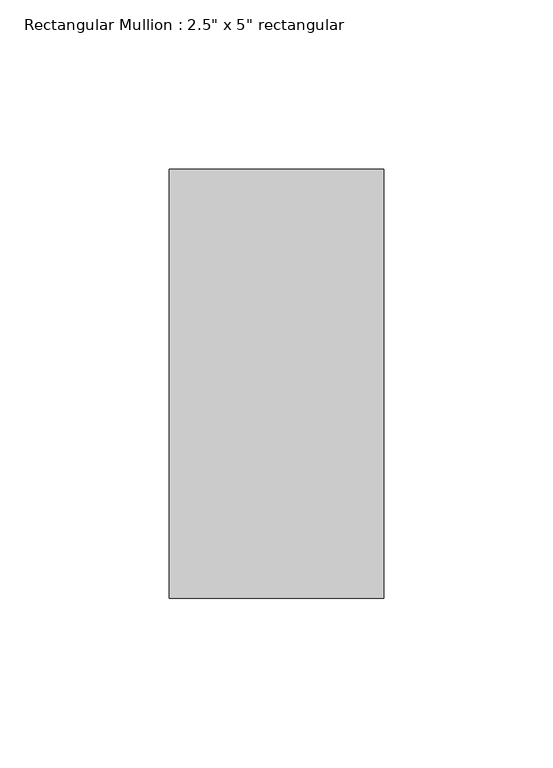
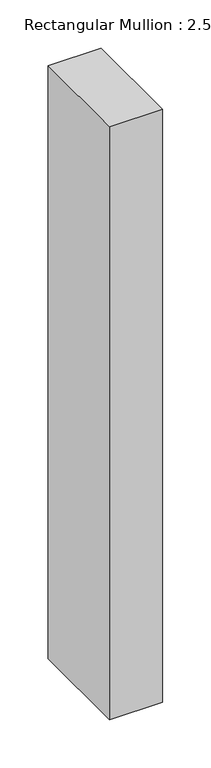
"""IFC4 building model written with IfcOpenShell, lengths in millimetres: member geometry."""

from ifc_helpers import new_model, si_unit, frame, origin, place, context, project, spatial, polyline, outline, extrude, source, transform, mapped, element, save


def member_798d6cad(model_context):
    return source(origin(), model_context, "Body", "SweptSolid", [
        extrude(outline(polyline([(31.75, 63.5), (31.75, -63.5), (-31.75, -63.5), (-31.75, 63.5), (31.75, 63.5)])), frame((0.0, 0.0, -749.3), z_axis=(0.0, 0.0, 1.0), x_axis=(1.0, 0.0, 0.0)), (0.0, 0.0, 1.0), 749.3),
    ])


if __name__ == "__main__":
    model = new_model("IFC4")
    model_context = context("Model", 3, world=origin())
    ifc_project = project(units=[si_unit("LENGTHUNIT", "METRE", prefix="MILLI")], contexts=[model_context])
    site = spatial("IfcSite", under=ifc_project)
    building = spatial("IfcBuilding", under=site)
    placement = place(None, origin())
    member_shape = member_798d6cad(model_context)
    element("IfcMember", 1, ObjectType="Rectangular Mullion : 2.5\" x 5\" rectangular", at=placement, inside=building, context=model_context, shape_type="MappedRepresentation", body=[
        mapped(member_shape, transform((0.0, 0.0, 0.0), x_axis=(1.0, 0.0, 0.0), y_axis=(0.0, 1.0, 0.0), z_axis=(0.0, 0.0, 1.0))),
    ])
    save(model, "model.ifc")

# Revit data of these elements
# Type "Rectangular Mullion : 2.5\" x 5\" rectangular"
#   built-in parameter 1007304 = 0.416667 (stored number, unit not read)
#   built-in parameter 1007301 = 0.104167 (stored number, unit not read)
#   built-in parameter 1007300 = 0.104167 (stored number, unit not read)
# Element 1 (IfcMember, "Rectangular Mullion : 2.5\" x 5\" rectangular")
#   Materials on its faces: "Aluminum"
# Materials
#   "Aluminum": class "Metal", colour RGB 247 247 247, transparency 0, Description = "Aluminum 6061", Cost = 0
